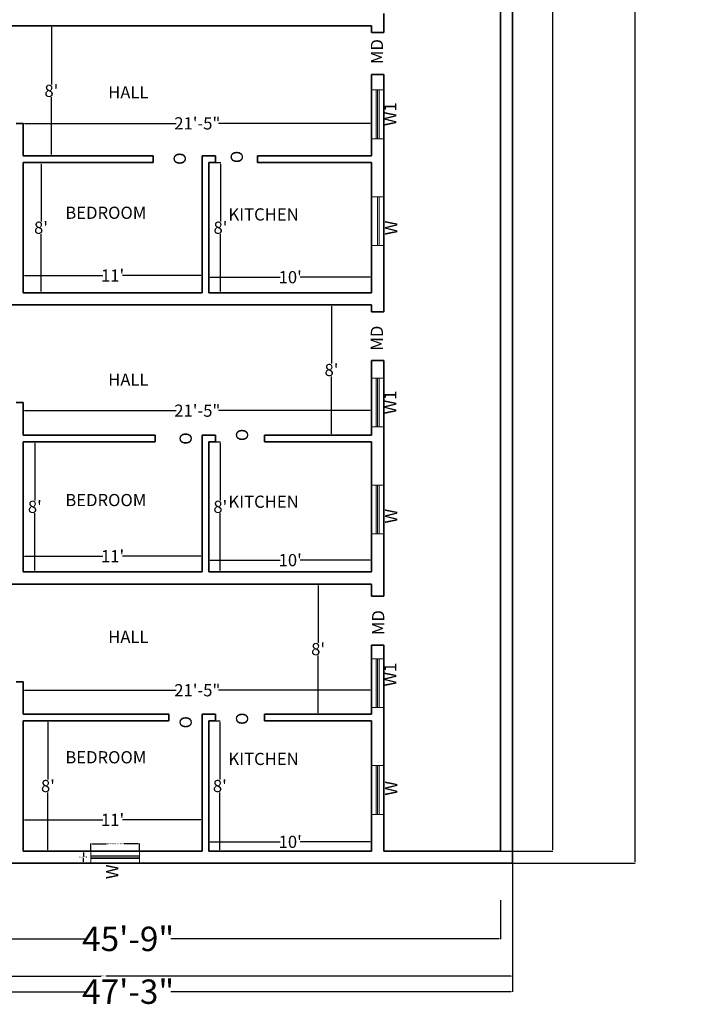
# Model space of a CAD drawing. Units: inches. Extents: x -2189 to 546, y 945 to 2684.
# Tile 2 of 10: x -626 to -134, y 945 to 1672. Entities that reach past the tile are written whole.
import ezdxf

# ---------------------------------------------------------------- set-up
doc = ezdxf.new("R2010")
doc.units = ezdxf.units.IN
doc.header["$MEASUREMENT"] = 0
for name, color, linetype, lineweight in [('A-ANNO-DIMS', 2, 'Continuous', 13), ('A-ANNO-TEXT', 7, 'Continuous', 18), ('A-AREA-IDEN', 3, 'Continuous', 18), ('A-GLAZ', 4, 'Continuous', 18), ('A-WALL', 7, 'Continuous', 35)]:
    doc.layers.add(name, color=color, linetype=linetype, lineweight=lineweight)
doc.styles.get("Standard").update_dxf_attribs({"font": 'arial.ttf'})
doc.dimstyles.get("Standard").update_dxf_attribs({"dimtxt": 1, "dimasz": 1, "dimexe": 0.18, "dimexo": 0.0625, "dimgap": 0.09, "dimtad": 0, "dimtih": 1, "dimtoh": 1, "dimdec": 0, "dimzin": 0, "dimdsep": 46, "dimlunit": 3, "dimtxsty": 'Standard', "dimcen": 0.09, "dimadec": 0, "dimazin": 0, "dimtfac": 1, "dimtdec": 0, "dimtofl": 0, "dimtmove": 0, "dimatfit": 3, "dimfxl": 1, "dimtolj": 1, "dimtzin": 0, "dimarcsym": 0})

# ---------------------------------------------------------------- blocks, each defined once
blk = doc.blocks.new('*D3')
at = {"layer": 'A-ANNO-DIMS', "color": 0, "lineweight": -2, "transparency": 16777216}
for p, q in [((-623.72, 1154.17), (-605.29, 1154.17)), ((-605.47, 1153.17), (-605.47, 1110.86)), ((-605.47, 1059.17), (-605.47, 1101.49)), ((-623.72, 1058.17), (-605.29, 1058.17))]:
    blk.add_line(p, q, dxfattribs=at)
at = {"layer": 'A-ANNO-DIMS', "color": 0, "transparency": 16777216}
for points in [[(-605.63, 1153.17), (-605.3, 1153.17), (-605.47, 1154.17)], [(-605.63, 1059.17), (-605.3, 1059.17), (-605.47, 1058.17)]]:
    blk.add_solid(points, dxfattribs=at)
at = {"layer": 'Defpoints', "color": 0, "transparency": 16777216}
for p in [(-623.78, 1154.17), (-605.47, 1154.17), (-623.78, 1058.17)]:
    blk.add_point(p, dxfattribs=at)
at = {"layer": 'A-ANNO-DIMS', "color": 0, "transparency": 16777216, "insert": (-605.47, 1106.17), "char_height": 1, "attachment_point": 5}
blk.add_mtext("\\A1;{\\H9x;8'}", dxfattribs=at)
blk = doc.blocks.new('*D4')
at = {"layer": 'A-ANNO-DIMS', "color": 0, "lineweight": -2, "transparency": 16777216}
for p, q in [((-623.78, 1058.24), (-623.78, 1081.42)), ((-622.78, 1081.24), (-565.08, 1081.24)), ((-492.78, 1081.24), (-550.48, 1081.24)), ((-491.78, 1058.24), (-491.78, 1081.42))]:
    blk.add_line(p, q, dxfattribs=at)
at = {"layer": 'A-ANNO-DIMS', "color": 0, "transparency": 16777216}
for points in [[(-622.78, 1081.4), (-622.78, 1081.07), (-623.78, 1081.24)], [(-492.78, 1081.4), (-492.78, 1081.07), (-491.78, 1081.24)]]:
    blk.add_solid(points, dxfattribs=at)
at = {"layer": 'Defpoints', "color": 0, "transparency": 16777216}
for p in [(-491.78, 1081.24), (-623.78, 1058.17), (-491.78, 1058.17)]:
    blk.add_point(p, dxfattribs=at)
at = {"layer": 'A-ANNO-DIMS', "color": 0, "transparency": 16777216, "insert": (-557.78, 1081.24), "char_height": 1, "attachment_point": 5}
blk.add_mtext("\\A1;{\\H9x;11'}", dxfattribs=at)
blk = doc.blocks.new('*D5')
at = {"layer": 'A-ANNO-DIMS', "color": 0, "lineweight": -2, "transparency": 16777216}
for p, q in [((-484.22, 1154.17), (-478.5, 1154.17)), ((-478.68, 1153.17), (-478.68, 1110.86)), ((-478.68, 1059.17), (-478.68, 1101.49)), ((-484.22, 1058.17), (-478.5, 1058.17))]:
    blk.add_line(p, q, dxfattribs=at)
at = {"layer": 'A-ANNO-DIMS', "color": 0, "transparency": 16777216}
for points in [[(-478.84, 1153.17), (-478.51, 1153.17), (-478.68, 1154.17)], [(-478.84, 1059.17), (-478.51, 1059.17), (-478.68, 1058.17)]]:
    blk.add_solid(points, dxfattribs=at)
at = {"layer": 'Defpoints', "color": 0, "transparency": 16777216}
for p in [(-484.28, 1154.17), (-484.28, 1058.17), (-478.68, 1058.17)]:
    blk.add_point(p, dxfattribs=at)
at = {"layer": 'A-ANNO-DIMS', "color": 0, "transparency": 16777216, "insert": (-478.68, 1106.17), "char_height": 1, "attachment_point": 5}
blk.add_mtext("\\A1;{\\H9x;8'}", dxfattribs=at)
blk = doc.blocks.new('*D6')
at = {"layer": 'A-ANNO-DIMS', "color": 0, "lineweight": -2, "transparency": 16777216}
for p, q in [((-486.78, 1058.24), (-486.78, 1065.15)), ((-485.78, 1064.97), (-434.08, 1064.97)), ((-367.78, 1064.97), (-419.48, 1064.97)), ((-366.78, 1058.24), (-366.78, 1065.15))]:
    blk.add_line(p, q, dxfattribs=at)
at = {"layer": 'A-ANNO-DIMS', "color": 0, "transparency": 16777216}
for points in [[(-485.78, 1065.14), (-485.78, 1064.81), (-486.78, 1064.97)], [(-367.78, 1065.14), (-367.78, 1064.81), (-366.78, 1064.97)]]:
    blk.add_solid(points, dxfattribs=at)
at = {"layer": 'Defpoints', "color": 0, "transparency": 16777216}
for p in [(-366.78, 1064.97), (-486.78, 1058.17), (-366.78, 1058.17)]:
    blk.add_point(p, dxfattribs=at)
at = {"layer": 'A-ANNO-DIMS', "color": 0, "transparency": 16777216, "insert": (-426.78, 1064.97), "char_height": 1, "attachment_point": 5}
blk.add_mtext("\\A1;{\\H9x;10'}", dxfattribs=at)
blk = doc.blocks.new('*D7')
at = {"layer": 'A-ANNO-DIMS', "color": 0, "lineweight": -2, "transparency": 16777216}
for p, q in [((-623.78, 1159.24), (-623.78, 1177.03)), ((-622.78, 1176.85), (-510.9, 1176.85)), ((-367.78, 1176.85), (-479.65, 1176.85)), ((-366.78, 1159.24), (-366.78, 1177.03))]:
    blk.add_line(p, q, dxfattribs=at)
at = {"layer": 'A-ANNO-DIMS', "color": 0, "transparency": 16777216}
for points in [[(-622.78, 1177.02), (-622.78, 1176.68), (-623.78, 1176.85)], [(-367.78, 1177.02), (-367.78, 1176.68), (-366.78, 1176.85)]]:
    blk.add_solid(points, dxfattribs=at)
at = {"layer": 'Defpoints', "color": 0, "transparency": 16777216}
for p in [(-366.78, 1176.85), (-623.78, 1159.17), (-366.78, 1159.17)]:
    blk.add_point(p, dxfattribs=at)
at = {"layer": 'A-ANNO-DIMS', "color": 0, "transparency": 16777216, "insert": (-495.28, 1176.85), "char_height": 1, "attachment_point": 5}
blk.add_mtext('\\A1;{\\H9x;21\'-5"}', dxfattribs=at)
blk = doc.blocks.new('*D8')
at = {"layer": 'A-ANNO-DIMS', "color": 0, "lineweight": -2, "transparency": 16777216}
for p, q in [((-366.84, 1255.17), (-406.38, 1255.17)), ((-406.2, 1254.17), (-406.2, 1211.86)), ((-406.2, 1160.17), (-406.2, 1202.49)), ((-366.84, 1159.17), (-406.38, 1159.17))]:
    blk.add_line(p, q, dxfattribs=at)
at = {"layer": 'A-ANNO-DIMS', "color": 0, "transparency": 16777216}
for points in [[(-406.37, 1254.17), (-406.04, 1254.17), (-406.2, 1255.17)], [(-406.37, 1160.17), (-406.04, 1160.17), (-406.2, 1159.17)]]:
    blk.add_solid(points, dxfattribs=at)
at = {"layer": 'Defpoints', "color": 0, "transparency": 16777216}
for p in [(-366.78, 1255.17), (-406.2, 1159.17), (-366.78, 1159.17)]:
    blk.add_point(p, dxfattribs=at)
at = {"layer": 'A-ANNO-DIMS', "color": 0, "transparency": 16777216, "insert": (-406.2, 1207.17), "char_height": 1, "attachment_point": 5}
blk.add_mtext("\\A1;{\\H9x;8'}", dxfattribs=at)
blk = doc.blocks.new('*D19')
at = {"layer": 'A-ANNO-DIMS', "color": 0, "lineweight": -2, "transparency": 16777216}
for p, q in [((-623.72, 1360.17), (-614.95, 1360.17)), ((-615.13, 1359.17), (-615.13, 1316.86)), ((-615.13, 1265.17), (-615.13, 1307.49)), ((-623.72, 1264.17), (-614.95, 1264.17))]:
    blk.add_line(p, q, dxfattribs=at)
at = {"layer": 'A-ANNO-DIMS', "color": 0, "transparency": 16777216}
for points in [[(-615.29, 1359.17), (-614.96, 1359.17), (-615.13, 1360.17)], [(-615.29, 1265.17), (-614.96, 1265.17), (-615.13, 1264.17)]]:
    blk.add_solid(points, dxfattribs=at)
at = {"layer": 'Defpoints', "color": 0, "transparency": 16777216}
for p in [(-623.78, 1360.17), (-615.13, 1360.17), (-623.78, 1264.17)]:
    blk.add_point(p, dxfattribs=at)
at = {"layer": 'A-ANNO-DIMS', "color": 0, "transparency": 16777216, "insert": (-615.13, 1312.17), "char_height": 1, "attachment_point": 5}
blk.add_mtext("\\A1;{\\H9x;8'}", dxfattribs=at)
blk = doc.blocks.new('*D20')
at = {"layer": 'A-ANNO-DIMS', "color": 0, "lineweight": -2, "transparency": 16777216}
for p, q in [((-623.78, 1264.24), (-623.78, 1275.94)), ((-622.78, 1275.76), (-565.08, 1275.76)), ((-492.78, 1275.76), (-550.48, 1275.76)), ((-491.78, 1264.24), (-491.78, 1275.94))]:
    blk.add_line(p, q, dxfattribs=at)
at = {"layer": 'A-ANNO-DIMS', "color": 0, "transparency": 16777216}
for points in [[(-622.78, 1275.92), (-622.78, 1275.59), (-623.78, 1275.76)], [(-492.78, 1275.92), (-492.78, 1275.59), (-491.78, 1275.76)]]:
    blk.add_solid(points, dxfattribs=at)
at = {"layer": 'Defpoints', "color": 0, "transparency": 16777216}
for p in [(-491.78, 1275.76), (-623.78, 1264.17), (-491.78, 1264.17)]:
    blk.add_point(p, dxfattribs=at)
at = {"layer": 'A-ANNO-DIMS', "color": 0, "transparency": 16777216, "insert": (-557.78, 1275.76), "char_height": 1, "attachment_point": 5}
blk.add_mtext("\\A1;{\\H9x;11'}", dxfattribs=at)
blk = doc.blocks.new('*D21')
at = {"layer": 'A-ANNO-DIMS', "color": 0, "lineweight": -2, "transparency": 16777216}
for p, q in [((-486.72, 1360.17), (-478.15, 1360.17)), ((-478.33, 1359.17), (-478.33, 1316.86)), ((-478.33, 1265.17), (-478.33, 1307.49)), ((-486.72, 1264.17), (-478.15, 1264.17))]:
    blk.add_line(p, q, dxfattribs=at)
at = {"layer": 'A-ANNO-DIMS', "color": 0, "transparency": 16777216}
for points in [[(-478.49, 1359.17), (-478.16, 1359.17), (-478.33, 1360.17)], [(-478.49, 1265.17), (-478.16, 1265.17), (-478.33, 1264.17)]]:
    blk.add_solid(points, dxfattribs=at)
at = {"layer": 'Defpoints', "color": 0, "transparency": 16777216}
for p in [(-486.78, 1360.17), (-478.33, 1360.17), (-486.78, 1264.17)]:
    blk.add_point(p, dxfattribs=at)
at = {"layer": 'A-ANNO-DIMS', "color": 0, "transparency": 16777216, "insert": (-478.33, 1312.17), "char_height": 1, "attachment_point": 5}
blk.add_mtext("\\A1;{\\H9x;8'}", dxfattribs=at)
blk = doc.blocks.new('*D22')
at = {"layer": 'A-ANNO-DIMS', "color": 0, "lineweight": -2, "transparency": 16777216}
for p, q in [((-486.78, 1264.24), (-486.78, 1273.01)), ((-485.78, 1272.83), (-434.08, 1272.83)), ((-367.78, 1272.83), (-419.48, 1272.83)), ((-366.78, 1264.24), (-366.78, 1273.01))]:
    blk.add_line(p, q, dxfattribs=at)
at = {"layer": 'A-ANNO-DIMS', "color": 0, "transparency": 16777216}
for points in [[(-485.78, 1273), (-485.78, 1272.66), (-486.78, 1272.83)], [(-367.78, 1273), (-367.78, 1272.66), (-366.78, 1272.83)]]:
    blk.add_solid(points, dxfattribs=at)
at = {"layer": 'Defpoints', "color": 0, "transparency": 16777216}
for p in [(-486.78, 1272.83), (-486.78, 1264.17), (-366.78, 1264.17)]:
    blk.add_point(p, dxfattribs=at)
at = {"layer": 'A-ANNO-DIMS', "color": 0, "transparency": 16777216, "insert": (-426.78, 1272.83), "char_height": 1, "attachment_point": 5}
blk.add_mtext("\\A1;{\\H9x;10'}", dxfattribs=at)
blk = doc.blocks.new('*D23')
at = {"layer": 'A-ANNO-DIMS', "color": 0, "lineweight": -2, "transparency": 16777216}
for p, q in [((-623.78, 1377.24), (-623.78, 1383.36)), ((-622.78, 1383.18), (-510.9, 1383.18)), ((-367.78, 1383.18), (-479.65, 1383.18)), ((-366.78, 1377.24), (-366.78, 1383.36))]:
    blk.add_line(p, q, dxfattribs=at)
at = {"layer": 'A-ANNO-DIMS', "color": 0, "transparency": 16777216}
for points in [[(-622.78, 1383.35), (-622.78, 1383.02), (-623.78, 1383.18)], [(-367.78, 1383.35), (-367.78, 1383.02), (-366.78, 1383.18)]]:
    blk.add_solid(points, dxfattribs=at)
at = {"layer": 'Defpoints', "color": 0, "transparency": 16777216}
for p in [(-366.78, 1383.18), (-623.78, 1377.17), (-366.78, 1377.17)]:
    blk.add_point(p, dxfattribs=at)
at = {"layer": 'A-ANNO-DIMS', "color": 0, "transparency": 16777216, "insert": (-495.28, 1383.18), "char_height": 1, "attachment_point": 5}
blk.add_mtext('\\A1;{\\H9x;21\'-5"}', dxfattribs=at)
blk = doc.blocks.new('*D24')
at = {"layer": 'A-ANNO-DIMS', "color": 0, "lineweight": -2, "transparency": 16777216}
for p, q in [((-406.22, 1461.17), (-396.17, 1461.17)), ((-396.35, 1460.17), (-396.35, 1417.86)), ((-396.35, 1366.17), (-396.35, 1408.49)), ((-406.22, 1365.17), (-396.17, 1365.17))]:
    blk.add_line(p, q, dxfattribs=at)
at = {"layer": 'A-ANNO-DIMS', "color": 0, "transparency": 16777216}
for points in [[(-396.51, 1460.17), (-396.18, 1460.17), (-396.35, 1461.17)], [(-396.51, 1366.17), (-396.18, 1366.17), (-396.35, 1365.17)]]:
    blk.add_solid(points, dxfattribs=at)
at = {"layer": 'Defpoints', "color": 0, "transparency": 16777216}
for p in [(-406.28, 1461.17), (-396.35, 1461.17), (-406.28, 1365.17)]:
    blk.add_point(p, dxfattribs=at)
at = {"layer": 'A-ANNO-DIMS', "color": 0, "transparency": 16777216, "insert": (-396.35, 1413.17), "char_height": 1, "attachment_point": 5}
blk.add_mtext("\\A1;{\\H9x;8'}", dxfattribs=at)
blk = doc.blocks.new('*D31')
at = {"layer": 'A-ANNO-DIMS', "color": 0, "lineweight": -2, "transparency": 16777216}
for p, q in [((-623.78, 1470.24), (-623.78, 1483.07)), ((-622.78, 1482.89), (-565.08, 1482.89)), ((-492.78, 1482.89), (-550.48, 1482.89)), ((-491.78, 1470.24), (-491.78, 1483.07))]:
    blk.add_line(p, q, dxfattribs=at)
at = {"layer": 'A-ANNO-DIMS', "color": 0, "transparency": 16777216}
for points in [[(-622.78, 1483.06), (-622.78, 1482.72), (-623.78, 1482.89)], [(-492.78, 1483.06), (-492.78, 1482.72), (-491.78, 1482.89)]]:
    blk.add_solid(points, dxfattribs=at)
at = {"layer": 'Defpoints', "color": 0, "transparency": 16777216}
for p in [(-491.78, 1482.89), (-623.78, 1470.17), (-491.78, 1470.17)]:
    blk.add_point(p, dxfattribs=at)
at = {"layer": 'A-ANNO-DIMS', "color": 0, "transparency": 16777216, "insert": (-557.78, 1482.89), "char_height": 1, "attachment_point": 5}
blk.add_mtext("\\A1;{\\H9x;11'}", dxfattribs=at)
blk = doc.blocks.new('*D32')
at = {"layer": 'A-ANNO-DIMS', "color": 0, "lineweight": -2, "transparency": 16777216}
for p, q in [((-623.72, 1566.17), (-610.39, 1566.17)), ((-610.57, 1565.17), (-610.57, 1522.86)), ((-610.57, 1471.17), (-610.57, 1513.49)), ((-623.72, 1470.17), (-610.39, 1470.17))]:
    blk.add_line(p, q, dxfattribs=at)
at = {"layer": 'A-ANNO-DIMS', "color": 0, "transparency": 16777216}
for points in [[(-610.74, 1565.17), (-610.41, 1565.17), (-610.57, 1566.17)], [(-610.74, 1471.17), (-610.41, 1471.17), (-610.57, 1470.17)]]:
    blk.add_solid(points, dxfattribs=at)
at = {"layer": 'Defpoints', "color": 0, "transparency": 16777216}
for p in [(-623.78, 1566.17), (-623.78, 1470.17), (-610.57, 1470.17)]:
    blk.add_point(p, dxfattribs=at)
at = {"layer": 'A-ANNO-DIMS', "color": 0, "transparency": 16777216, "insert": (-610.57, 1518.17), "char_height": 1, "attachment_point": 5}
blk.add_mtext("\\A1;{\\H9x;8'}", dxfattribs=at)
blk = doc.blocks.new('*D33')
at = {"layer": 'A-ANNO-DIMS', "color": 0, "lineweight": -2, "transparency": 16777216}
for p, q in [((-486.72, 1566.17), (-478.05, 1566.17)), ((-478.23, 1565.17), (-478.23, 1522.86)), ((-478.23, 1471.17), (-478.23, 1513.49)), ((-486.72, 1470.17), (-478.05, 1470.17))]:
    blk.add_line(p, q, dxfattribs=at)
at = {"layer": 'A-ANNO-DIMS', "color": 0, "transparency": 16777216}
for points in [[(-478.4, 1565.17), (-478.07, 1565.17), (-478.23, 1566.17)], [(-478.4, 1471.17), (-478.07, 1471.17), (-478.23, 1470.17)]]:
    blk.add_solid(points, dxfattribs=at)
at = {"layer": 'Defpoints', "color": 0, "transparency": 16777216}
for p in [(-486.78, 1566.17), (-478.23, 1566.17), (-486.78, 1470.17)]:
    blk.add_point(p, dxfattribs=at)
at = {"layer": 'A-ANNO-DIMS', "color": 0, "transparency": 16777216, "insert": (-478.23, 1518.17), "char_height": 1, "attachment_point": 5}
blk.add_mtext("\\A1;{\\H9x;8'}", dxfattribs=at)
blk = doc.blocks.new('*D34')
at = {"layer": 'A-ANNO-DIMS', "color": 0, "lineweight": -2, "transparency": 16777216}
for p, q in [((-486.78, 1470.24), (-486.78, 1481.84)), ((-485.78, 1481.66), (-434.08, 1481.66)), ((-367.78, 1481.66), (-419.48, 1481.66)), ((-366.78, 1470.24), (-366.78, 1481.84))]:
    blk.add_line(p, q, dxfattribs=at)
at = {"layer": 'A-ANNO-DIMS', "color": 0, "transparency": 16777216}
for points in [[(-485.78, 1481.83), (-485.78, 1481.5), (-486.78, 1481.66)], [(-367.78, 1481.83), (-367.78, 1481.5), (-366.78, 1481.66)]]:
    blk.add_solid(points, dxfattribs=at)
at = {"layer": 'Defpoints', "color": 0, "transparency": 16777216}
for p in [(-366.78, 1481.66), (-486.78, 1470.17), (-366.78, 1470.17)]:
    blk.add_point(p, dxfattribs=at)
at = {"layer": 'A-ANNO-DIMS', "color": 0, "transparency": 16777216, "insert": (-426.78, 1481.66), "char_height": 1, "attachment_point": 5}
blk.add_mtext("\\A1;{\\H9x;10'}", dxfattribs=at)
blk = doc.blocks.new('*D35')
at = {"layer": 'A-ANNO-DIMS', "color": 0, "lineweight": -2, "transparency": 16777216}
for p, q in [((-623.72, 1667.17), (-602.74, 1667.17)), ((-602.92, 1666.17), (-602.92, 1623.86)), ((-602.92, 1572.17), (-602.92, 1614.49)), ((-623.72, 1571.17), (-602.74, 1571.17))]:
    blk.add_line(p, q, dxfattribs=at)
at = {"layer": 'A-ANNO-DIMS', "color": 0, "transparency": 16777216}
for points in [[(-603.09, 1666.17), (-602.75, 1666.17), (-602.92, 1667.17)], [(-603.09, 1572.17), (-602.75, 1572.17), (-602.92, 1571.17)]]:
    blk.add_solid(points, dxfattribs=at)
at = {"layer": 'Defpoints', "color": 0, "transparency": 16777216}
for p in [(-623.78, 1667.17), (-602.92, 1667.17), (-623.78, 1571.17)]:
    blk.add_point(p, dxfattribs=at)
at = {"layer": 'A-ANNO-DIMS', "color": 0, "transparency": 16777216, "insert": (-602.92, 1619.17), "char_height": 1, "attachment_point": 5}
blk.add_mtext("\\A1;{\\H9x;8'}", dxfattribs=at)
blk = doc.blocks.new('*D36')
at = {"layer": 'A-ANNO-DIMS', "color": 0, "lineweight": -2, "transparency": 16777216}
for p, q in [((-623.78, 1586.31), (-623.78, 1595.35)), ((-622.78, 1595.17), (-510.9, 1595.17)), ((-367.78, 1595.17), (-479.65, 1595.17)), ((-366.78, 1586.31), (-366.78, 1595.35))]:
    blk.add_line(p, q, dxfattribs=at)
at = {"layer": 'A-ANNO-DIMS', "color": 0, "transparency": 16777216}
for points in [[(-622.78, 1595.34), (-622.78, 1595.01), (-623.78, 1595.17)], [(-367.78, 1595.34), (-367.78, 1595.01), (-366.78, 1595.17)]]:
    blk.add_solid(points, dxfattribs=at)
at = {"layer": 'Defpoints', "color": 0, "transparency": 16777216}
for p in [(-366.78, 1595.17), (-623.78, 1586.25), (-366.78, 1586.25)]:
    blk.add_point(p, dxfattribs=at)
at = {"layer": 'A-ANNO-DIMS', "color": 0, "transparency": 16777216, "insert": (-495.28, 1595.17), "char_height": 1, "attachment_point": 5}
blk.add_mtext('\\A1;{\\H9x;21\'-5"}', dxfattribs=at)
blk = doc.blocks.new('*D79')
at = {"layer": 'A-ANNO-DIMS', "color": 0, "lineweight": -2, "transparency": 16777216}
for p, q in [((-262.72, 2600.17), (-172.26, 2600.17)), ((-172.44, 2599.17), (-172.44, 1833.96)), ((-172.44, 1050.17), (-172.44, 1815.39)), ((-262.72, 1049.17), (-172.26, 1049.17))]:
    blk.add_line(p, q, dxfattribs=at)
at = {"layer": 'A-ANNO-DIMS', "color": 0, "transparency": 16777216}
for points in [[(-172.6, 2599.17), (-172.27, 2599.17), (-172.44, 2600.17)], [(-172.6, 1050.17), (-172.27, 1050.17), (-172.44, 1049.17)]]:
    blk.add_solid(points, dxfattribs=at)
at = {"layer": 'Defpoints', "color": 0, "transparency": 16777216}
for p in [(-262.78, 2600.17), (-172.44, 2600.17), (-262.78, 1049.17)]:
    blk.add_point(p, dxfattribs=at)
at = {"layer": 'A-ANNO-DIMS', "color": 0, "transparency": 16777216, "insert": (-172.44, 1824.67), "char_height": 1, "attachment_point": 5}
blk.add_mtext('\\A1;{\\H18x;129\'-3"}', dxfattribs=at)
blk = doc.blocks.new('*D80')
at = {"layer": 'A-ANNO-DIMS', "color": 0, "lineweight": -2, "transparency": 16777216}
for p, q in [((-271.72, 2591.17), (-233.01, 2591.17)), ((-233.19, 2590.17), (-233.19, 1833.95)), ((-233.19, 1059.17), (-233.19, 1815.39)), ((-271.72, 1058.17), (-233.01, 1058.17))]:
    blk.add_line(p, q, dxfattribs=at)
at = {"layer": 'A-ANNO-DIMS', "color": 0, "transparency": 16777216}
for points in [[(-233.36, 2590.17), (-233.03, 2590.17), (-233.19, 2591.17)], [(-233.36, 1059.17), (-233.03, 1059.17), (-233.19, 1058.17)]]:
    blk.add_solid(points, dxfattribs=at)
at = {"layer": 'Defpoints', "color": 0, "transparency": 16777216}
for p in [(-271.78, 2591.17), (-233.19, 2591.17), (-271.78, 1058.17)]:
    blk.add_point(p, dxfattribs=at)
at = {"layer": 'A-ANNO-DIMS', "color": 0, "transparency": 16777216, "insert": (-233.19, 1824.67), "char_height": 1, "attachment_point": 5}
blk.add_mtext('\\A1;{\\H18x;127\'-9"}', dxfattribs=at)
blk = doc.blocks.new('*D81')
at = {"layer": 'A-ANNO-DIMS', "color": 0, "lineweight": -2, "transparency": 16777216}
for p, q in [((-829.78, 1049.11), (-829.78, 954.22)), ((-262.78, 1049.11), (-262.78, 954.22)), ((-828.78, 954.4), (-577.65, 954.4)), ((-263.78, 954.4), (-514.91, 954.4))]:
    blk.add_line(p, q, dxfattribs=at)
at = {"layer": 'A-ANNO-DIMS', "color": 0, "transparency": 16777216}
for points in [[(-828.78, 954.57), (-828.78, 954.24), (-829.78, 954.4)], [(-263.78, 954.57), (-263.78, 954.24), (-262.78, 954.4)]]:
    blk.add_solid(points, dxfattribs=at)
at = {"layer": 'Defpoints', "color": 0, "transparency": 16777216}
for p in [(-829.78, 1049.17), (-262.78, 1049.17), (-262.78, 954.4)]:
    blk.add_point(p, dxfattribs=at)
at = {"layer": 'A-ANNO-DIMS', "color": 0, "transparency": 16777216, "insert": (-546.28, 954.4), "char_height": 1, "attachment_point": 5}
blk.add_mtext('\\A1;{\\H18x;47\'-3"}', dxfattribs=at)
blk = doc.blocks.new('*D82')
at = {"layer": 'A-ANNO-DIMS', "color": 0, "lineweight": -2, "transparency": 16777216}
for p, q in [((-820.78, 1021.94), (-820.78, 993.18)), ((-271.78, 1021.94), (-271.78, 993.18)), ((-819.78, 993.36), (-577.65, 993.36)), ((-272.78, 993.36), (-514.91, 993.36))]:
    blk.add_line(p, q, dxfattribs=at)
at = {"layer": 'A-ANNO-DIMS', "color": 0, "transparency": 16777216}
for points in [[(-819.78, 993.52), (-819.78, 993.19), (-820.78, 993.36)], [(-272.78, 993.52), (-272.78, 993.19), (-271.78, 993.36)]]:
    blk.add_solid(points, dxfattribs=at)
at = {"layer": 'Defpoints', "color": 0, "transparency": 16777216}
for p in [(-820.78, 1022), (-271.78, 1022), (-271.78, 993.36)]:
    blk.add_point(p, dxfattribs=at)
at = {"layer": 'A-ANNO-DIMS', "color": 0, "transparency": 16777216, "insert": (-546.28, 993.36), "char_height": 1, "attachment_point": 5}
blk.add_mtext('\\A1;{\\H18x;45\'-9"}', dxfattribs=at)
blk = doc.blocks.new('WIN-36X9')
for p, q in [((0, 5.5), (36, 5.5)), ((0, 5.5), (36, 5.5)), ((0, 4.5), (36, 4.5)), ((0, 3.5), (36, 3.5))]:
    blk.add_line(p, q)
blk.add_lwpolyline([(0, 0), (0, 9), (36, 9), (36, 0)], close=True)
blk = doc.blocks.new('WIN-36X9-TWINLINE')
for p, q in [((4.5, 0), (4.5, 36)), ((5.5, 0), (5.5, 36))]:
    blk.add_line(p, q)
blk.add_lwpolyline([(9, 0), (0, 0), (0, 36), (9, 36)], close=True)
blk = doc.blocks.new('*D91')
at = {"layer": 'A-ANNO-DIMS', "color": 0, "lineweight": -2, "transparency": 16777216}
for p, q in [((-573.87, 1058.24), (-573.87, 1063.75)), ((-572.87, 1063.57), (-562.29, 1063.57)), ((-538.87, 1063.57), (-549.46, 1063.57)), ((-537.87, 1058.24), (-537.87, 1063.75))]:
    blk.add_line(p, q, dxfattribs=at)
at = {"layer": 'A-ANNO-DIMS', "color": 0, "transparency": 16777216}
for points in [[(-572.87, 1063.74), (-572.87, 1063.41), (-573.87, 1063.57)], [(-538.87, 1063.74), (-538.87, 1063.41), (-537.87, 1063.57)]]:
    blk.add_solid(points, dxfattribs=at)
at = {"layer": 'Defpoints', "color": 0, "transparency": 16777216}
for p in [(-537.87, 1063.57), (-573.87, 1058.17), (-537.87, 1058.17)]:
    blk.add_point(p, dxfattribs=at)
at = {"layer": 'A-ANNO-DIMS', "color": 0, "transparency": 16777216, "insert": (-555.87, 1063.57), "char_height": 1, "attachment_point": 5}
blk.add_mtext('\\A1;WINDOW 3\'-0" TYP.', dxfattribs=at)
blk = doc.blocks.new('*D92')
at = {"layer": 'A-ANNO-DIMS', "color": 0, "lineweight": -2, "transparency": 16777216}
for p, q in [((-573.94, 1058.17), (-579.45, 1058.17)), ((-579.27, 1057.17), (-579.27, 1054.27)), ((-573.94, 1049.17), (-579.45, 1049.17)), ((-579.27, 1050.17), (-579.27, 1053.07))]:
    blk.add_line(p, q, dxfattribs=at)
at = {"layer": 'A-ANNO-DIMS', "color": 0, "transparency": 16777216}
for points in [[(-579.44, 1057.17), (-579.11, 1057.17), (-579.27, 1058.17)], [(-579.44, 1050.17), (-579.11, 1050.17), (-579.27, 1049.17)]]:
    blk.add_solid(points, dxfattribs=at)
at = {"layer": 'Defpoints', "color": 0, "transparency": 16777216}
for p in [(-579.27, 1058.17), (-573.87, 1058.17), (-573.87, 1049.17)]:
    blk.add_point(p, dxfattribs=at)
at = {"layer": 'A-ANNO-DIMS', "color": 0, "transparency": 16777216, "insert": (-579.27, 1053.67), "char_height": 1, "attachment_point": 5}
blk.add_mtext('\\A1;0\'-9" TYP.', dxfattribs=at)
blk = doc.blocks.new('*D103')
at = {"layer": 'A-ANNO-DIMS', "color": 0, "lineweight": -2, "transparency": 16777216}
for p, q in [((-865.78, 1070.94), (-865.78, 965.69)), ((-262.78, 1049.11), (-262.78, 965.69)), ((-864.78, 965.87), (-566.09, 965.87)), ((-263.78, 965.87), (-562.47, 965.87))]:
    blk.add_line(p, q, dxfattribs=at)
at = {"layer": 'A-ANNO-DIMS', "color": 0, "transparency": 16777216}
for points in [[(-864.78, 966.04), (-864.78, 965.71), (-865.78, 965.87)], [(-263.78, 966.04), (-263.78, 965.71), (-262.78, 965.87)]]:
    blk.add_solid(points, dxfattribs=at)
at = {"layer": 'Defpoints', "color": 0, "transparency": 16777216}
for p in [(-865.78, 1071.01), (-262.78, 1049.17), (-262.78, 965.87)]:
    blk.add_point(p, dxfattribs=at)
at = {"layer": 'A-ANNO-DIMS', "color": 0, "transparency": 16777216, "insert": (-564.28, 965.87), "char_height": 1, "attachment_point": 5}
blk.add_mtext('\\A1;50\'-3"', dxfattribs=at)

msp = doc.modelspace()

# ---------------------------------------------------------------- linework, layer by layer
at = {"layer": 'A-WALL'}
for p, q in [((-262.78, 2600.17), (-262.78, 1049.17)), ((-271.78, 2591.17), (-271.78, 1058.17)), ((-357.78, 1662.17), (-357.78, 1676.17)), ((-366.78, 1667.17), (-695.78, 1667.17)), ((-366.78, 1662.17), (-366.78, 1667.17)), ((-366.78, 1662.17), (-357.78, 1662.17)), ((-366.78, 1631.17), (-357.78, 1631.17)), ((-366.78, 1571.17), (-366.78, 1631.17)), ((-357.78, 1456.17), (-357.78, 1631.17)), ((-623.78, 1595.17), (-628.78, 1595.17)), ((-623.78, 1571.17), (-623.78, 1595.17)), ((-534.63, 1571.17), (-623.78, 1571.17)), ((-527.78, 1571.17), (-623.78, 1571.17)), ((-527.78, 1566.17), (-527.78, 1571.17)), ((-491.78, 1470.17), (-491.78, 1571.17)), ((-481.78, 1571.17), (-491.78, 1571.17)), ((-481.78, 1566.17), (-481.78, 1571.17)), ((-366.78, 1571.17), (-450.78, 1571.17)), ((-450.78, 1566.17), (-450.78, 1571.17)), ((-623.78, 1470.17), (-623.78, 1566.17)), ((-527.78, 1566.17), (-623.78, 1566.17)), ((-486.78, 1470.17), (-486.78, 1566.17)), ((-481.78, 1566.17), (-486.78, 1566.17)), ((-366.78, 1566.17), (-450.78, 1566.17)), ((-366.78, 1470.17), (-366.78, 1566.17)), ((-491.78, 1470.17), (-623.78, 1470.17)), ((-366.78, 1470.17), (-486.78, 1470.17)), ((-623.78, 1461.17), (-690.78, 1461.17)), ((-366.78, 1461.17), (-623.78, 1461.17)), ((-491.78, 1461.17), (-623.78, 1461.17)), ((-366.78, 1456.17), (-366.78, 1461.17)), ((-366.78, 1456.17), (-357.78, 1456.17)), ((-366.78, 1365.17), (-366.78, 1420.17)), ((-366.78, 1420.17), (-357.78, 1420.17)), ((-357.78, 1246.17), (-357.78, 1420.17)), ((-623.78, 1389.17), (-628.78, 1389.17)), ((-623.78, 1365.17), (-623.78, 1389.17)), ((-526.44, 1365.17), (-623.78, 1365.17)), ((-623.78, 1264.17), (-623.78, 1360.17)), ((-526.44, 1360.17), (-623.78, 1360.17)), ((-526.44, 1365.17), (-526.44, 1360.17)), ((-491.78, 1264.17), (-491.78, 1365.17)), ((-481.78, 1365.17), (-491.78, 1365.17)), ((-481.78, 1365.17), (-486.78, 1365.17)), ((-486.78, 1264.17), (-486.78, 1360.17)), ((-481.78, 1360.17), (-486.78, 1360.17)), ((-481.78, 1360.17), (-481.78, 1365.17)), ((-366.78, 1365.17), (-445.78, 1365.17)), ((-445.78, 1360.17), (-445.78, 1365.17)), ((-366.78, 1360.17), (-445.78, 1360.17)), ((-366.78, 1264.17), (-366.78, 1360.17)), ((-491.78, 1264.17), (-623.78, 1264.17)), ((-366.78, 1264.17), (-486.78, 1264.17)), ((-366.78, 1255.17), (-690.78, 1255.17)), ((-366.78, 1246.17), (-366.78, 1255.17)), ((-366.78, 1246.17), (-357.78, 1246.17)), ((-366.78, 1159.17), (-366.78, 1210.17)), ((-366.78, 1210.17), (-357.78, 1210.17)), ((-357.78, 1058.17), (-357.78, 1210.17)), ((-623.78, 1183.17), (-628.78, 1183.17)), ((-623.78, 1159.17), (-623.78, 1183.17)), ((-516.25, 1159.17), (-623.78, 1159.17)), ((-516.25, 1159.17), (-516.25, 1154.17)), ((-491.78, 1058.17), (-491.78, 1159.17)), ((-481.78, 1159.17), (-491.78, 1159.17)), ((-481.78, 1159.17), (-481.78, 1154.17)), ((-366.78, 1159.17), (-445.62, 1159.17)), ((-445.62, 1159.17), (-445.62, 1154.17)), ((-623.78, 1058.17), (-623.78, 1154.17)), ((-516.25, 1154.17), (-623.78, 1154.17)), ((-486.78, 1058.17), (-486.78, 1154.17)), ((-481.78, 1154.17), (-486.78, 1154.17)), ((-366.78, 1154.17), (-445.62, 1154.17)), ((-366.78, 1058.17), (-366.78, 1154.17)), ((-491.78, 1058.17), (-623.78, 1058.17)), ((-366.78, 1058.17), (-486.78, 1058.17)), ((-271.78, 1058.17), (-357.78, 1058.17)), ((-262.78, 1049.17), (-829.78, 1049.17))]:
    msp.add_line(p, q, dxfattribs=at)

# ---------------------------------------------------------------- block references
at = {"layer": 'A-GLAZ'}
for p, rotation in [((-357.78, 1583.85), 90.00000000000142), ((-357.78, 1371.12), 90.00000000000142), ((-357.78, 1292.28), 90.00000000000126), ((-357.78, 1164.07), 90.00000000000126), ((-357.78, 1085.23), 90.00000000000111)]:
    msp.add_blockref('WIN-36X9', p, dxfattribs=dict(at, rotation=rotation))
for name, p in [('WIN-36X9-TWINLINE', (-366.78, 1505.01)), ('WIN-36X9', (-573.87, 1049.17))]:
    msp.add_blockref(name, p, dxfattribs=at)

# ---------------------------------------------------------------- texts
at = {"layer": 'A-ANNO-TEXT', "char_height": 9, "attachment_point": 1, "rotation": 90}
for s, width, heights, insert in [('MD', 16.482, [0], (-367.28, 1638.95)), ('W1', 11.3125, [0], (-357.59, 1593.12)), ('O', 18.6541, [0.207], (-512.78, 1564.57)), ('O', 18.6541, [0.207], (-470.67, 1565.84)), ('W', 11.3125, [0], (-356.83, 1512.63)), ('MD', 16.482, [0], (-367.35, 1427.5)), ('W1', 11.3125, [0], (-357.59, 1380.39)), ('O', 18.6541, [0.207], (-508.38, 1358.05)), ('O', 18.6541, [0.207], (-466.79, 1360.68)), ('W', 11.3125, [0], (-356.83, 1299.9)), ('MD', 16.482, [0], (-366.38, 1217.54)), ('W1', 11.3125, [0], (-357.59, 1179.55)), ('O', 18.6541, [0.207], (-508.38, 1148.66)), ('O', 18.6541, [0.207], (-466.79, 1151.29)), ('W', 11.3125, [0], (-356.83, 1099.06)), ('W', 11.3125, [0], (-562.55, 1037.49))]:
    msp.add_mtext_dynamic_manual_height_columns(s, width=width, gutter_width=1, heights=heights, dxfattribs=dict(at, insert=insert))
at = {"layer": 'A-AREA-IDEN', "char_height": 9, "attachment_point": 1}
for s, width, heights, insert in [('HALL', 37.3459, [0], (-561.01, 1622.54)), ('BEDROOM', 73.8205, [0.207], (-592.63, 1533.7)), ('KITCHEN', 69.371, [0], (-472.3, 1532.48)), ('HALL', 37.3459, [0], (-561.01, 1410.53)), ('BEDROOM', 73.8205, [0.207], (-592.63, 1321.69)), ('KITCHEN', 69.371, [0], (-472.3, 1320.47)), ('HALL', 37.3459, [0], (-561.01, 1220.73)), ('BEDROOM', 73.8205, [0.207], (-592.63, 1131.89)), ('KITCHEN', 69.371, [0], (-472.3, 1130.67))]:
    msp.add_mtext_dynamic_manual_height_columns(s, width=width, gutter_width=1, heights=heights, dxfattribs=dict(at, insert=insert))

# ---------------------------------------------------------------- dimensions: what is measured, and where the dimension line sits
at = {"layer": 'A-ANNO-DIMS'}
for base, p1, p2, angle, text, override, picture, middle in [((-172.44, 2600.17), (-262.78, 1049.17), (-262.78, 2600.17), 90, '{\\H18x;<>}', {"dimclrd": 0, "dimclre": 0, "dimclrt": 0}, '*D79', (-172.44, 1824.67)), ((-233.19, 2591.17), (-271.78, 1058.17), (-271.78, 2591.17), 90, '{\\H18x;<>}', {"dimclrd": 0, "dimclre": 0, "dimclrt": 0}, '*D80', (-233.19, 1824.67)), ((-602.92, 1667.17), (-623.78, 1571.17), (-623.78, 1667.17), 90, '{\\H9x;<>}', {"dimclrd": 0, "dimclre": 0, "dimclrt": 0}, '*D35', (-602.92, 1619.17)), ((-366.78, 1595.17), (-623.78, 1586.25), (-366.78, 1586.25), 180, '{\\H9x;<>}', {"dimclrd": 0, "dimclre": 0, "dimclrt": 0}, '*D36', (-495.28, 1595.17)), ((-610.57, 1470.17), (-623.78, 1566.17), (-623.78, 1470.17), 90, '{\\H9x;<>}', {"dimclrd": 0, "dimclre": 0, "dimclrt": 0}, '*D32', (-610.57, 1518.17)), ((-478.23, 1566.17), (-486.78, 1470.17), (-486.78, 1566.17), 90, '{\\H9x;<>}', {"dimclrd": 0, "dimclre": 0, "dimclrt": 0}, '*D33', (-478.23, 1518.17)), ((-491.78, 1482.89), (-623.78, 1470.17), (-491.78, 1470.17), 180, '{\\H9x;<>}', {"dimclrd": 0, "dimclre": 0, "dimclrt": 0}, '*D31', (-557.78, 1482.89)), ((-366.78, 1481.66), (-486.78, 1470.17), (-366.78, 1470.17), 180, '{\\H9x;<>}', {"dimclrd": 0, "dimclre": 0, "dimclrt": 0}, '*D34', (-426.78, 1481.66)), ((-396.35, 1461.17), (-406.28, 1365.17), (-406.28, 1461.17), 90, '{\\H9x;<>}', {"dimclrd": 0, "dimclre": 0, "dimclrt": 0}, '*D24', (-396.35, 1413.17)), ((-366.78, 1383.18), (-623.78, 1377.17), (-366.78, 1377.17), 180, '{\\H9x;<>}', {"dimclrd": 0, "dimclre": 0, "dimclrt": 0}, '*D23', (-495.28, 1383.18)), ((-615.13, 1360.17), (-623.78, 1264.17), (-623.78, 1360.17), 90, '{\\H9x;<>}', {"dimclrd": 0, "dimclre": 0, "dimclrt": 0}, '*D19', (-615.13, 1312.17)), ((-478.33, 1360.17), (-486.78, 1264.17), (-486.78, 1360.17), 90, '{\\H9x;<>}', {"dimclrd": 0, "dimclre": 0, "dimclrt": 0}, '*D21', (-478.33, 1312.17)), ((-491.78, 1275.76), (-623.78, 1264.17), (-491.78, 1264.17), 180, '{\\H9x;<>}', {"dimclrd": 0, "dimclre": 0, "dimclrt": 0}, '*D20', (-557.78, 1275.76)), ((-486.78, 1272.83), (-366.78, 1264.17), (-486.78, 1264.17), 180, '{\\H9x;<>}', {"dimclrd": 0, "dimclre": 0, "dimclrt": 0}, '*D22', (-426.78, 1272.83)), ((-406.2, 1159.17), (-366.78, 1255.17), (-366.78, 1159.17), 90, '{\\H9x;<>}', {"dimclrd": 0, "dimclre": 0, "dimclrt": 0}, '*D8', (-406.2, 1207.17)), ((-605.47, 1154.17), (-623.78, 1058.17), (-623.78, 1154.17), 90, '{\\H9x;<>}', {"dimclrd": 0, "dimclre": 0, "dimclrt": 0}, '*D3', (-605.47, 1106.17)), ((-478.68, 1058.17), (-484.28, 1154.17), (-484.28, 1058.17), 90, '{\\H9x;<>}', {"dimclrd": 0, "dimclre": 0, "dimclrt": 0}, '*D5', (-478.68, 1106.17)), ((-579.27, 1058.17), (-573.87, 1049.17), (-573.87, 1058.17), 90, '<> TYP.', {"dimdec": 1, "dimlfac": 1, "dimrnd": 0, "dimzin": 1, "dimdsep": 46, "dimlunit": 4, "dimfrac": 2}, '*D92', (-579.27, 1053.67))]:
    dim = msp.add_linear_dim(base=base, p1=p1, p2=p2, angle=angle, text=text, dimstyle='Standard', override=override, dxfattribs=at)
    dim.commit()
    dim.dimension.update_dxf_attribs({"geometry": picture, "text_midpoint": middle})
for base, p1, p2, text, override, picture, middle in [((-366.78, 1176.85), (-623.78, 1159.17), (-366.78, 1159.17), '{\\H9x;<>}', {"dimclrd": 0, "dimclre": 0, "dimclrt": 0}, '*D7', (-495.28, 1176.85)), ((-491.78, 1081.24), (-623.78, 1058.17), (-491.78, 1058.17), '{\\H9x;<>}', {"dimclrd": 0, "dimclre": 0, "dimclrt": 0}, '*D4', (-557.78, 1081.24)), ((-366.78, 1064.97), (-486.78, 1058.17), (-366.78, 1058.17), '{\\H9x;<>}', {"dimclrd": 0, "dimclre": 0, "dimclrt": 0}, '*D6', (-426.78, 1064.97)), ((-537.87, 1063.57), (-573.87, 1058.17), (-537.87, 1058.17), 'WINDOW <> TYP.', {"dimdec": 1, "dimlfac": 1, "dimrnd": 0, "dimzin": 1, "dimdsep": 46, "dimlunit": 4, "dimfrac": 2}, '*D91', (-555.87, 1063.57)), ((-262.78, 954.4), (-829.78, 1049.17), (-262.78, 1049.17), '{\\H18x;<>}', {"dimclrd": 0, "dimclre": 0, "dimclrt": 0}, '*D81', (-546.28, 954.4)), ((-271.78, 993.36), (-820.78, 1022), (-271.78, 1022), '{\\H18x;<>}', {"dimclrd": 0, "dimclre": 0, "dimclrt": 0}, '*D82', (-546.28, 993.36))]:
    dim = msp.add_linear_dim(base=base, p1=p1, p2=p2, text=text, dimstyle='Standard', override=override, dxfattribs=at)
    dim.commit()
    dim.dimension.update_dxf_attribs({"geometry": picture, "text_midpoint": middle})
dim = msp.add_linear_dim(base=(-262.78, 965.87), p1=(-865.78, 1071.01), p2=(-262.78, 1049.17), dimstyle='Standard', override={"dimdec": 1, "dimlfac": 1, "dimrnd": 0, "dimzin": 1, "dimdsep": 46, "dimlunit": 4, "dimfrac": 2}, dxfattribs=at)
dim.commit()
dim.dimension.update_dxf_attribs({"geometry": '*D103', "text_midpoint": (-564.28, 965.87)})

doc.saveas('drawing.dxf')
